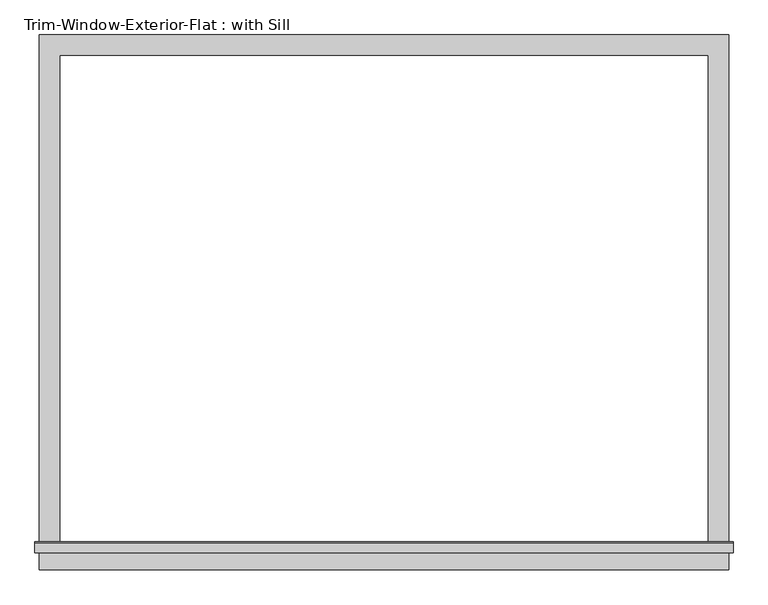
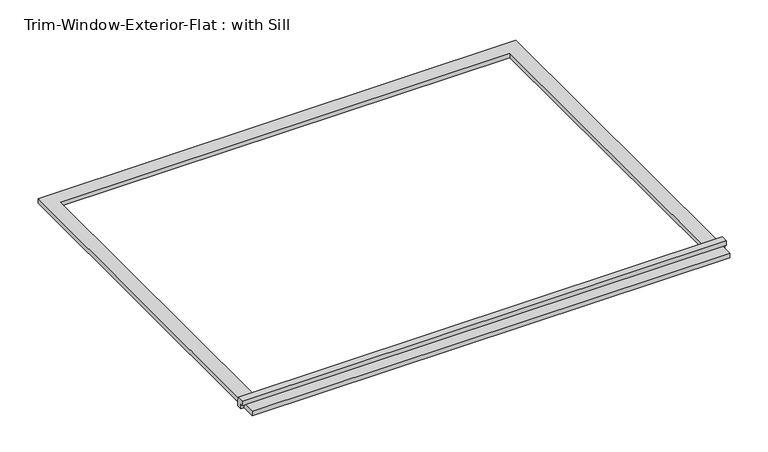
"""IFC4 building model written with IfcOpenShell, lengths in millimetres: proxy geometry, Trim-Window-Exterior-Flat : with Sill."""

from ifc_helpers import new_model, si_unit, frame, origin, origin_with_axes, place, context, project, spatial, polyline, outline, extrude, source, transform, mapped, element, save


def trim_window_exterior_flat_with_sill_3212bfb3(model_context):
    return source(origin(), model_context, "Body", "SweptSolid", [
        extrude(outline(polyline([(971.55, -1393.7823709), (971.55, -1450.9323709), (-971.55, -1450.9323709), (-971.55, -1393.7823709), (971.55, -1393.7823709)])), origin_with_axes(), (0.0, 0.0, 1.0), 19.05),
        extrude(outline(polyline([(-1403.35, 38.1), (-1374.0580645, 38.1), (-1371.6, 19.05), (-1371.6, 0.0), (-1393.7823709, 0.0), (-1393.7823709, 19.05), (-1403.35, 19.05), (-1403.35, 38.1)])), frame((-984.25, 0.0, 0.0), z_axis=(1.0, 0.0, 0.0), x_axis=(0.0, 1.0, 0.0)), (0.0, 0.0, 1.0), 1968.5),
        extrude(outline(polyline([(-971.55, 57.15), (971.55, 57.15), (971.55, -1371.6), (914.4, -1371.6), (914.4, 0.0), (-914.4, 0.0), (-914.4, -1371.6), (-971.55, -1371.6), (-971.55, 57.15)])), origin_with_axes(), (0.0, 0.0, 1.0), 19.05),
    ])


if __name__ == "__main__":
    model = new_model("IFC4")
    model_context = context("Model", 3, world=origin())
    ifc_project = project(units=[si_unit("LENGTHUNIT", "METRE", prefix="MILLI")], contexts=[model_context])
    site = spatial("IfcSite", under=ifc_project)
    building = spatial("IfcBuilding", under=site)
    placement = place(None, origin())
    trim_window_exterior_flat_with_sill_shape = trim_window_exterior_flat_with_sill_3212bfb3(model_context)
    element("IfcBuildingElementProxy", 1, Name="Trim-Window-Exterior-Flat : with Sill", ObjectType="Trim-Window-Exterior-Flat : with Sill", at=placement, inside=building, context=model_context, shape_type="MappedRepresentation", body=[
        mapped(trim_window_exterior_flat_with_sill_shape, transform((0.0, 0.0, 0.0), x_axis=(1.0, 0.0, 0.0), y_axis=(0.0, 1.0, 0.0), z_axis=(0.0, 0.0, 1.0))),
    ])
    save(model, "model.ifc")

# Revit data of these elements
# Type "Trim-Window-Exterior-Flat : with Sill"
#   Trim Width = 0' - 2 1/4"
#   Trim Thickness_Picture Frame = 0' - 1 1/4"
#   Trim Thickness_with Sill = 0' - 0 3/4"
#   Sill Thickness = 0' - 1 1/4"
#   Opening Width [instance default] = 2' - 0"
#   Opening Height [instance default] = 3' - 0"
#   Default Elevation = 4' - 0"
#   Sill = yes
#   Picture Frame = no
#   Trim Material [instance default] = none
# Element 1 (IfcBuildingElementProxy, "Trim-Window-Exterior-Flat : with Sill")
#   Opening Width = 6' - 0"
#   Opening Height = 4' - 6"
#   Trim Material = Clad - White
#   Materials on its faces: "Clad - White"
# Materials
#   "Clad - White": class "Wood", colour RGB 242 242 238, transparency 0, Cost = 0
